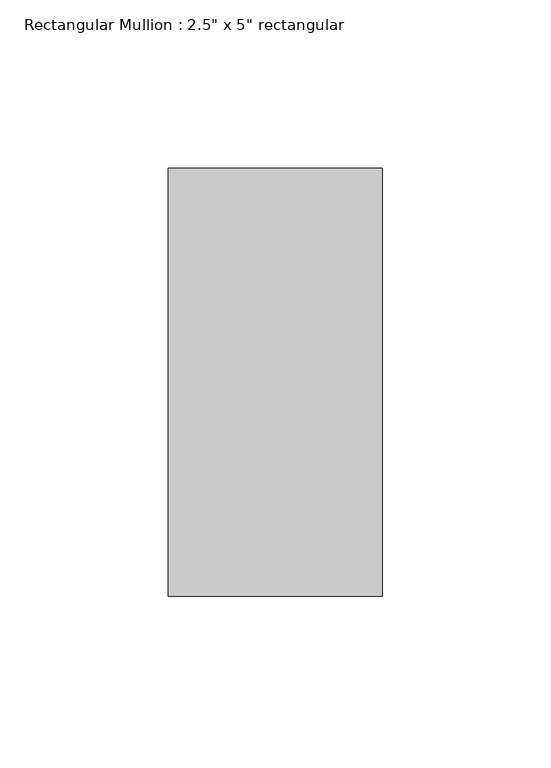
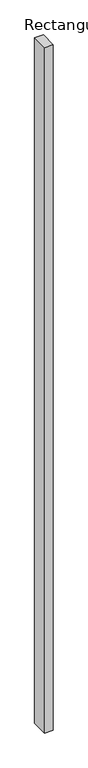
"""IFC4 building model written with IfcOpenShell, lengths in millimetres: member geometry."""

from ifc_helpers import new_model, si_unit, frame, origin, place, context, project, spatial, polyline, outline, extrude, source, transform, mapped, element, save


def member_e8a6e381(model_context):
    return source(origin(), model_context, "Body", "SweptSolid", [
        extrude(outline(polyline([(0.0, 63.5), (0.0, -63.5), (-63.5, -63.5), (-63.5, 63.5), (0.0, 63.5)])), frame((0.0, 0.0, -5353.05), z_axis=(0.0, 0.0, 1.0), x_axis=(1.0, 0.0, 0.0)), (0.0, 0.0, 1.0), 5353.05),
    ])


if __name__ == "__main__":
    model = new_model("IFC4")
    model_context = context("Model", 3, world=origin())
    ifc_project = project(units=[si_unit("LENGTHUNIT", "METRE", prefix="MILLI")], contexts=[model_context])
    site = spatial("IfcSite", under=ifc_project)
    building = spatial("IfcBuilding", under=site)
    placement = place(None, origin())
    member_shape = member_e8a6e381(model_context)
    element("IfcMember", 1, ObjectType="Rectangular Mullion : 2.5\" x 5\" rectangular", at=placement, inside=building, context=model_context, shape_type="MappedRepresentation", body=[
        mapped(member_shape, transform((0.0, 0.0, 0.0), x_axis=(1.0, 0.0, 0.0), y_axis=(0.0, 1.0, 0.0), z_axis=(0.0, 0.0, 1.0))),
    ])
    save(model, "model.ifc")

# Revit data of these elements
# Type "Rectangular Mullion : 2.5\" x 5\" rectangular"
#   built-in parameter 1007304 = 0.416667 (stored number, unit not read)
#   built-in parameter 1007301 = 0.104167 (stored number, unit not read)
#   built-in parameter 1007300 = 0.104167 (stored number, unit not read)
# Element 1 (IfcMember, "Rectangular Mullion : 2.5\" x 5\" rectangular")
#   Materials on its faces: "Aluminum"
# Materials
#   "Aluminum": class "Metal", colour RGB 247 247 247, transparency 0, Description = "Aluminum 6061", Cost = 0
